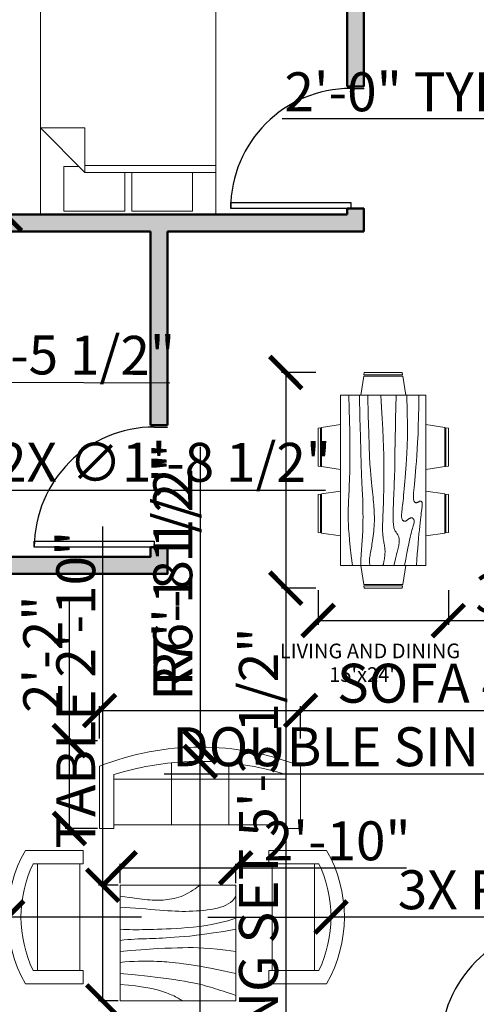
# Model space of a CAD drawing. Units: inches. Extents: x 3147 to 3847, y 1414 to 2207.
# Tile 3 of 7: x 3437 to 3572, y 1561 to 1852. Entities that reach past the tile are written whole.
import ezdxf

# ---------------------------------------------------------------- set-up
doc = ezdxf.new("R2010")
doc.units = ezdxf.units.IN
for name, color, linetype, lineweight in [('A-ANNO-DIMS', 2, 'Continuous', 18), ('A-AREA-IDEN', 7, 'Continuous', 18), ('A-DOOR', 3, 'Continuous', 25), ('A-FURN', 8, 'Continuous', 18), ('A-WALL', 7, 'Continuous', 50)]:
    doc.layers.add(name, color=color, linetype=linetype, lineweight=lineweight)
doc.layers.add('A-WALL-PATT', color=18, linetype='Continuous', lineweight=13, true_color=0x000000)
doc.styles.get("Standard").update_dxf_attribs({"font": 'arial.ttf'})
doc.dimstyles.new('ISO-25', dxfattribs={"dimtxt": 11.5, "dimasz": 9.5, "dimexe": 1.25, "dimexo": 0.625, "dimtad": 1, "dimdec": 0, "dimlunit": 3, "dimtxsty": 'Standard', "dimblk": 'ARCHTICK', "dimcen": 2.5, "dimadec": 0, "dimazin": 0, "dimtfac": 1, "dimtdec": 0, "dimtmove": 0, "dimatfit": 3, "dimfxl": 1, "dimarcsym": 0})

# ---------------------------------------------------------------- blocks, each defined once
blk = doc.blocks.new('*U6')
for p, q in [((0, 0), (0, -100)), ((900, 0), (900, -100))]:
    blk.add_line(p, q)
blk.add_lwpolyline([(0, 0), (0, 900), (43.75, 900), (43.75, 0)], close=True)
blk.add_arc((0, 0), 900, 0, 90)
blk = doc.blocks.new('Sofa - Roundback 7 ft.')
for p, q in [((-12.00002, -32.4421), (-12.00003, -6.5971)), ((11.99997, -32.4421), (11.99998, -6.5971)), ((-36.000027, -34), (-36.000027, -11.4696)), ((35.99998, -34), (35.99998, -11.4696)), ((-35.999844, -13.3819), (35.9998, -13.3819)), ((-36.000027, -32.4421), (35.99998, -32.4421))]:
    blk.add_line(p, q)
for points in [[(-36.000027, -34), (-42.000027, -34), (-42.000027, -8)], [(41.99998, -8), (41.99998, -34), (35.99998, -34)]]:
    blk.add_lwpolyline(points)
for centre, radius, start, end in [((0, -114.25), 114.25, 68.43141, 111.5686), ((-0.00001, -127.1968), 121.1968, 72.72033, 107.2797)]:
    blk.add_arc(centre, radius, start, end)
blk = doc.blocks.new('Table - Square Woodgrain 42 x 42 in.')
blk.add_line((0, -42), (42, -42))
for points in [[(0, -4), (1.704, -4.2172), (3.2358, -4.4188), (4.615, -4.604), (5.8615, -4.7721), (6.9951, -4.9224), (8.0357, -5.0541), (9.0031, -5.1667), (9.9171, -5.2594), (10.7951, -5.3316), (11.6445, -5.3836), (12.4702, -5.4157), (13.277, -5.4283), (14.0698, -5.4217), (14.8535, -5.3964), (15.6331, -5.3526), (16.4133, -5.2908), (17.1986, -5.2103), (17.9913, -5.1062), (18.793, -4.9727), (19.6056, -4.8038), (20.4307, -4.5937), (21.2701, -4.3365), (22.1256, -4.0262), (22.9989, -3.6571), (23.888, -3.2272), (24.7756, -2.7516), (25.6408, -2.2491), (26.4624, -1.7387), (27.2195, -1.2395), (27.891, -0.7703), (28.456, -0.3501), (28.8934, 0.002)], [(0, -42), (0, 0), (42, 0), (42, -42)], [(0, -8), (1.8203, -8.1001), (3.6741, -8.2149), (5.5411, -8.3408), (7.4011, -8.4741), (9.2339, -8.6112), (11.0193, -8.7484), (12.7371, -8.8821), (14.3671, -9.0086), (15.8954, -9.1246), (17.3337, -9.2278), (18.6997, -9.3159), (20.0116, -9.387), (21.2871, -9.4389), (22.5442, -9.4696), (23.8008, -9.477), (25.0749, -9.459), (26.3791, -9.4137), (27.7049, -9.3403), (29.0383, -9.2382), (30.3655, -9.1068), (31.6728, -8.9455), (32.9461, -8.7535), (34.1717, -8.5304), (35.3358, -8.2756), (36.4268, -7.9863), (37.443, -7.6521), (38.3849, -7.2603), (39.253, -6.7986), (40.048, -6.2542), (40.7705, -5.6147), (41.421, -4.8674), (42, -4)], [(42, -12), (39.1784, -12.8621), (36.4519, -13.5654), (33.8246, -14.1294), (31.3004, -14.5731), (28.8832, -14.9161), (26.577, -15.1775), (24.3858, -15.3768), (22.3136, -15.5332), (20.3622, -15.6632), (18.5254, -15.7718), (16.7947, -15.8612), (15.1618, -15.9338), (13.6183, -15.9916), (12.1558, -16.0369), (10.7659, -16.0718), (9.4403, -16.0987), (8.1703, -16.1191), (6.9461, -16.1325), (5.7577, -16.1377), (4.595, -16.1335), (3.4479, -16.1188), (2.3064, -16.0924), (1.1604, -16.0532), (0, -16)], [(42, -16), (37.6529, -16.7365), (33.8802, -17.329), (30.6179, -17.7961), (27.8015, -18.1561), (25.3668, -18.4275), (23.2497, -18.6288), (21.3859, -18.7785), (19.7111, -18.8949), (18.1693, -18.9939), (16.7375, -19.0795), (15.401, -19.1534), (14.1449, -19.217), (12.9544, -19.2717), (11.8148, -19.3191), (10.7113, -19.3606), (9.6291, -19.3976), (8.5534, -19.4323), (7.47, -19.4689), (6.3643, -19.5122), (5.222, -19.5672), (4.0288, -19.6386), (2.7703, -19.7313), (1.4321, -19.8501), (0, -20)], [(0, -24), (3.9243, -23.6805), (7.4766, -23.4138), (10.6891, -23.1954), (13.5943, -23.0205), (16.2247, -22.8847), (18.6125, -22.7832), (20.7903, -22.7116), (22.7903, -22.6651), (24.6563, -22.642), (26.4764, -22.6507), (28.35, -22.7024), (30.3766, -22.8084), (32.6555, -22.98), (35.2861, -23.2283), (38.3678, -23.5645), (42, -24)], [(42, -32), (37.392, -31.017), (33.4585, -30.2231), (30.1291, -29.5949), (27.3334, -29.109), (25.0009, -28.742), (23.0612, -28.4707), (21.4439, -28.2716), (20.0786, -28.1215), (18.8998, -28.0002), (17.8609, -27.9014), (16.9206, -27.8219), (16.0371, -27.7588), (15.1691, -27.709), (14.2748, -27.6693), (13.3128, -27.6368), (12.2415, -27.6083), (11.0295, -27.5824), (9.6867, -27.5643), (8.233, -27.5608), (6.6884, -27.5787), (5.0728, -27.6248), (3.4062, -27.7058), (1.7086, -27.8286), (0, -28)], [(0, -32), (5.4026, -32.5358), (9.9494, -33.019), (13.7424, -33.4553), (16.8834, -33.8505), (19.4743, -34.2106), (21.6171, -34.5413), (23.4136, -34.8486), (24.9657, -35.1382), (26.3614, -35.4156), (27.6332, -35.6841), (28.7995, -35.9467), (29.8788, -36.2064), (30.8897, -36.4661), (31.8507, -36.7288), (32.7802, -36.9973), (33.6968, -37.2747), (34.6175, -37.5635), (35.5531, -37.8651), (36.5128, -38.1805), (37.506, -38.5108), (38.5421, -38.8568), (39.6302, -39.2197), (40.7797, -39.6004), (42, -40)], [(0, -36), (3.0098, -36.2857), (5.5354, -36.5643), (7.6368, -36.8359), (9.374, -37.1009), (10.807, -37.3597), (11.9957, -37.6126), (13.0002, -37.8599), (13.8804, -38.102), (14.6874, -38.3393), (15.4365, -38.5729), (16.1338, -38.8041), (16.7858, -39.0341), (17.3987, -39.264), (17.9787, -39.4952), (18.5322, -39.7288), (19.0655, -39.9662), (19.5832, -40.2081), (20.0842, -40.4544), (20.5657, -40.7046), (21.0249, -40.9581), (21.459, -41.2144), (21.8653, -41.4731), (22.2409, -41.7335), (22.5831, -41.9951)]]:
    blk.add_lwpolyline(points)
blk = doc.blocks.new('Dining Set - 36 x 72 in.')
for p, q in [((-22.2343, 26.00059), (-23.4847, 17.99762)), ((-22.2304, 26), (-5.7608, 26)), ((-22, 27.5), (-22.1562, 26.50042)), ((-5.8416, 26.5), (-22.1534, 26.5)), ((-22, 27.5), (-6, 27.5)), ((-5.8437, 26.49966), (-6, 27.5)), ((-4.5152, 17.99762), (-5.7655, 25.99926)), ((5.7657, 26.00059), (4.5153, 17.99762)), ((5.7696, 26), (22.2392, 26)), ((6, 27.5), (5.8438, 26.50042)), ((22.1584, 26.5), (5.8466, 26.5)), ((6, 27.5), (22, 27.5)), ((22.1563, 26.49966), (22, 27.5)), ((23.4848, 17.99762), (22.2345, 25.99926)), ((36, 18), (-36, 18)), ((-36, 18), (-36, -18)), ((36, -18), (36, 18)), ((-44.0006, 8.23428), (-35.9976, 9.48474)), ((44.0006, 8.23428), (35.9976, 9.48474)), ((-45.5, 8), (-44.5004, 8.15617)), ((-45.5, 8), (-45.5, -8)), ((-44.5, -8.15843), (-44.5, 8.15338)), ((-44, 8.23041), (-44, -8.23915)), ((44, 8.23041), (44, -8.23915)), ((44.5, -8.15843), (44.5, 8.15338)), ((45.5, 8), (44.5005, 8.15617)), ((45.5, 8), (45.5, -8)), ((-44.4997, -8.15631), (-45.5, -8)), ((-35.9976, -9.48476), (-43.9993, -8.2345)), ((35.9976, -9.48476), (43.9993, -8.2345)), ((44.4997, -8.15631), (45.5, -8)), ((-36, -18), (36, -18)), ((-22.2343, -26.0006), (-23.4847, -17.99762)), ((-4.5152, -17.99762), (-5.7655, -25.99928)), ((5.7657, -26.0006), (4.5153, -17.99762)), ((23.4848, -17.99762), (22.2345, -25.99928)), ((-22.2304, -26), (-5.7608, -26)), ((-22, -27.5), (-22.1562, -26.50044)), ((-5.8416, -26.5), (-22.1534, -26.5)), ((-22, -27.5), (-6, -27.5)), ((-5.8437, -26.49967), (-6, -27.5)), ((5.7696, -26), (22.2392, -26)), ((6, -27.5), (5.8438, -26.50044)), ((22.1584, -26.5), (5.8466, -26.5)), ((6, -27.5), (22, -27.5)), ((22.1563, -26.49967), (22, -27.5))]:
    blk.add_line(p, q)
for points in [[(-36, 15), (-31.1772, 14.97754), (-26.8079, 14.91406), (-22.8538, 14.81543), (-19.276, 14.6875), (-16.0362, 14.53613), (-13.0957, 14.36718), (-10.4159, 14.18652), (-7.9583, 14), (-5.6904, 13.81315), (-3.6035, 13.63021), (-1.6954, 13.45508), (0.0365, 13.29166), (1.5945, 13.14388), (2.9811, 13.01562), (4.1988, 12.9108), (5.25, 12.83333), (6.1393, 12.78613), (6.8802, 12.76823), (7.4883, 12.77767), (7.9792, 12.8125), (8.3685, 12.87077), (8.6719, 12.95052), (8.9049, 13.0498), (9.0833, 13.16666), (9.2205, 13.29899), (9.3216, 13.44401), (9.3895, 13.59879), (9.4271, 13.76041), (9.4373, 13.92594), (9.4232, 14.09245), (9.3875, 14.257), (9.3333, 14.41666), (9.2638, 14.56917), (9.1836, 14.71484), (9.0975, 14.85465), (9.0104, 14.98958), (8.9272, 15.1206), (8.8529, 15.2487), (8.7922, 15.37483), (8.75, 15.5), (8.7305, 15.62467), (8.7344, 15.74739), (8.7617, 15.86621), (8.8125, 15.97916), (8.8867, 16.08431), (8.9844, 16.17968), (9.1055, 16.26334), (9.25, 16.33333), (9.4189, 16.38802), (9.6172, 16.42708), (9.8506, 16.45052), (10.125, 16.45833), (10.4463, 16.45052), (10.8203, 16.42708), (11.2529, 16.38802), (11.75, 16.33333), (12.3184, 16.26318), (12.9694, 16.17838), (13.7151, 16.07991), (14.5677, 15.96875), (15.5395, 15.84586), (16.6426, 15.71224), (17.8893, 15.56884), (19.2917, 15.41666), (20.859, 15.25667), (22.5879, 15.08984), (24.4721, 14.91715), (26.5052, 14.73958), (28.6809, 14.5581), (30.9929, 14.3737), (33.4347, 14.18733), (36, 14)], [(-36, 10), (-28.9766, 10.14274), (-23.1725, 10.20442), (-18.4241, 10.19775), (-14.5677, 10.13541), (-11.4399, 10.03011), (-8.877, 9.89453), (-6.7154, 9.74137), (-4.7917, 9.58333), (-2.9698, 9.43082), (-1.2246, 9.28515), (0.4415, 9.14534), (2.026, 9.01041), (3.5266, 8.87939), (4.9408, 8.7513), (6.266, 8.62516), (7.5, 8.5), (8.6411, 8.37549), (9.6914, 8.2539), (10.6538, 8.13818), (11.5312, 8.03125), (12.3267, 7.93603), (13.043, 7.85547), (13.6831, 7.79248), (14.25, 7.75), (14.7471, 7.7303), (15.1797, 7.73307), (15.5537, 7.75732), (15.875, 7.80208), (16.1494, 7.86637), (16.3828, 7.94922), (16.5811, 8.04964), (16.75, 8.16666), (16.8944, 8.29915), (17.0143, 8.44531), (17.1089, 8.60319), (17.1771, 8.77083), (17.218, 8.94629), (17.2305, 9.1276), (17.2137, 9.31282), (17.1667, 9.5), (17.0895, 9.6875), (16.987, 9.875), (16.8649, 10.0625), (16.7292, 10.25), (16.5856, 10.4375), (16.4401, 10.625), (16.2985, 10.8125), (16.1667, 11), (16.05, 11.18733), (15.9518, 11.3737), (15.8752, 11.5581), (15.8229, 11.73958), (15.798, 11.91715), (15.8034, 12.08984), (15.842, 12.25667), (15.9167, 12.41666), (16.0295, 12.56836), (16.1784, 12.70833), (16.3605, 12.83268), (16.5729, 12.9375), (16.8127, 13.01888), (17.0768, 13.07291), (17.3625, 13.0957), (17.6667, 13.08333), (17.9894, 13.03312), (18.3418, 12.94726), (18.7382, 12.82918), (19.1927, 12.68229), (19.7195, 12.51001), (20.3327, 12.31575), (21.0465, 12.10294), (21.875, 11.875), (22.8357, 11.63354), (23.959, 11.37304), (25.2786, 11.08618), (26.8282, 10.76562), (28.6414, 10.40405), (30.752, 9.99414), (33.1936, 9.52856), (36, 9)], [(-36, 5.5), (-30.7157, 5.3348), (-26.069, 5.20963), (-21.9946, 5.11767), (-18.4271, 5.05208), (-15.3009, 5.00602), (-12.5508, 4.97265), (-10.1112, 4.94515), (-7.9167, 4.91666), (-5.909, 4.88167), (-4.0586, 4.83984), (-2.3429, 4.79215), (-0.7396, 4.73958), (0.7739, 4.6831), (2.22, 4.6237), (3.6213, 4.56233), (5, 4.5), (6.373, 4.43782), (7.7344, 4.3776), (9.0723, 4.32129), (10.375, 4.27083), (11.6309, 4.22819), (12.8281, 4.19531), (13.9551, 4.17415), (15, 4.16666), (15.954, 4.17448), (16.819, 4.19791), (17.6001, 4.23698), (18.3021, 4.29166), (18.9299, 4.36198), (19.4883, 4.44791), (19.9823, 4.54948), (20.4167, 4.66666), (20.7969, 4.79899), (21.1302, 4.94401), (21.4245, 5.09879), (21.6875, 5.26041), (21.9271, 5.42594), (22.1511, 5.59245), (22.3672, 5.757), (22.5834, 5.91666), (22.8065, 6.06868), (23.0404, 6.21093), (23.2879, 6.34147), (23.5521, 6.45833), (23.8358, 6.55957), (24.142, 6.64323), (24.4735, 6.70735), (24.8334, 6.75), (25.2235, 6.76969), (25.642, 6.76692), (26.0858, 6.74267), (26.5521, 6.69791), (27.0379, 6.63362), (27.5404, 6.55078), (28.0565, 6.45036), (28.5834, 6.33333), (29.1242, 6.19987), (29.7071, 6.04687), (30.3661, 5.87044), (31.1354, 5.66666), (32.0493, 5.43164), (33.142, 5.16146), (34.4475, 4.85221), (36, 4.5)], [(-36, -1), (-30.7915, -0.6591), (-26.0195, -0.38216), (-21.6519, -0.16284), (-17.6563, 0.00521), (-14.0005, 0.12833), (-10.6523, 0.21289), (-7.5796, 0.26522), (-4.75, 0.29166), (-2.134, 0.29793), (0.2878, 0.28711), (2.5317, 0.26163), (4.6146, 0.22396), (6.5529, 0.17651), (8.3633, 0.12174), (10.0623, 0.06209), (11.6667, 0), (13.1899, -0.06201), (14.6341, -0.1211), (15.9982, -0.17432), (17.2813, -0.21875), (18.4823, -0.25147), (19.6003, -0.26953), (20.6343, -0.27002), (21.5834, -0.25), (22.4481, -0.20768), (23.2357, -0.14584), (23.9549, -0.06836), (24.6146, 0.02083), (25.2235, 0.11784), (25.7904, 0.21875), (26.3241, 0.31966), (26.8334, 0.41666), (27.3265, 0.50618), (27.8099, 0.58593), (28.2894, 0.65397), (28.7709, 0.70833), (29.2601, 0.74707), (29.763, 0.76823), (30.2855, 0.76985), (30.8334, 0.75), (31.4088, 0.70784), (31.9994, 0.64713), (32.589, 0.57275), (33.1615, 0.48958), (33.7008, 0.4025), (34.1908, 0.3164), (34.6153, 0.23616), (34.9584, 0.16666), (35.2099, 0.11165), (35.3848, 0.07031), (35.504, 0.04069), (35.5886, 0.02083), (35.6594, 0.00879), (35.7377, 0.0026), (35.8442, 0.00032), (36, 0)], [(-36, -6.5), (-27.1843, -6.31267), (-20.084, -6.1263), (-14.469, -5.9419), (-10.1094, -5.76042), (-6.7752, -5.58285), (-4.2363, -5.41016), (-2.2629, -5.24333), (-0.625, -5.08334), (0.8708, -4.93099), (2.2715, -4.78646), (3.5872, -4.64974), (4.8281, -4.52084), (6.0046, -4.39974), (7.127, -4.28646), (8.2053, -4.18099), (9.25, -4.08334), (10.2705, -3.99382), (11.2734, -3.91407), (12.2647, -3.84603), (13.25, -3.79167), (14.2354, -3.75293), (15.2266, -3.73177), (16.2295, -3.73015), (17.25, -3.75), (18.2912, -3.79248), (19.3451, -3.85547), (20.4009, -3.93604), (21.4479, -4.03125), (22.4754, -4.13819), (23.4727, -4.25391), (24.4289, -4.37549), (25.3334, -4.5), (26.1785, -4.62492), (26.9694, -4.74935), (27.7145, -4.87281), (28.4219, -4.99479), (29.1, -5.11483), (29.7572, -5.23242), (30.4016, -5.34709), (31.0417, -5.45834), (31.6837, -5.56437), (32.3262, -5.65821), (32.9658, -5.73153), (33.599, -5.77604), (34.2224, -5.78345), (34.8327, -5.74545), (35.4264, -5.65373), (36, -5.5)], [(-36, -10), (-26.4022, -9.81299), (-18.4675, -9.62891), (-11.9839, -9.45069), (-6.7396, -9.28125), (-2.5226, -9.12354), (0.8789, -8.98047), (3.6769, -8.85498), (6.0833, -8.75), (8.2767, -8.66765), (10.3021, -8.60677), (12.1712, -8.56543), (13.8958, -8.54167), (15.4876, -8.53353), (16.9583, -8.53907), (18.3197, -8.55632), (19.5834, -8.58334), (20.7616, -8.61841), (21.8685, -8.66081), (22.9188, -8.71004), (23.9271, -8.76563), (24.9081, -8.82707), (25.8763, -8.89388), (26.8465, -8.96558), (27.8334, -9.04167), (28.8474, -9.12118), (29.8828, -9.20117), (30.93, -9.27824), (31.9792, -9.34896), (33.0205, -9.40991), (34.0443, -9.45768), (35.0407, -9.48885), (36, -9.5)], [(-36, -14.5), (-30.0881, -14.33513), (-25.0332, -14.21224), (-20.7312, -14.12647), (-17.0781, -14.07292), (-13.97, -14.04671), (-11.3027, -14.04297), (-8.9724, -14.05681), (-6.875, -14.08334), (-4.9224, -14.11833), (-3.0905, -14.16016), (-1.3709, -14.20785), (0.2448, -14.26042), (1.7647, -14.3169), (3.1973, -14.3763), (4.5507, -14.43767), (5.8333, -14.5), (7.0554, -14.5621), (8.235, -14.62175), (9.3922, -14.67652), (10.5469, -14.72396), (11.7192, -14.76164), (12.929, -14.78711), (14.1965, -14.79794), (15.5417, -14.79167), (16.9933, -14.76424), (18.6152, -14.70508), (20.4804, -14.60197), (22.6615, -14.44271), (25.2312, -14.21509), (28.2624, -13.9069), (31.8277, -13.50594), (36, -13)]]:
    blk.add_lwpolyline(points)
blk = doc.blocks.new('Bed - Queen')
for p, q in [((0, -80.00003), (0, 0)), ((0, 0), (59.99999, 0)), ((59.99999, 0), (59.99999, -80.00003)), ((7.99999, -1.2), (28.79998, -1.2)), ((7.99999, -14.4), (7.99999, -1.2)), ((28.79998, -1.2), (28.79998, -14.4)), ((31.19999, -1.2), (51.99999, -1.2)), ((31.19999, -14.4), (31.19999, -1.2)), ((51.99999, -1.2), (51.99999, -16.4)), ((0, -14.4), (44.8, -14.4)), ((44.8, -16.8), (0, -16.8)), ((59.99999, -29.6), (44.8, -14.4)), ((44.8, -14.4), (44.8, -29.6)), ((51.99999, -16.4), (46.79936, -16.4)), ((44.8, -29.6), (59.99999, -29.6)), ((59.99999, -80.00003), (0, -80.00003))]:
    blk.add_line(p, q)
blk = doc.blocks.new('Sofa - Roundback Loveseat 5 ft.')
for p, q in [((0, -32.44198), (0, -5.99998)), ((-24, -33.99998), (-24, -11.46958)), ((24.00004, -33.99998), (24.00004, -11.46958)), ((-23.9998, -13.38178), (23.99986, -13.38178)), ((-24, -32.44198), (24.00004, -32.44198))]:
    blk.add_line(p, q)
for points in [[(-24, -33.99998), (-30, -33.99998), (-30, -7.99998)], [(30.00004, -7.99998), (30.00004, -33.99998), (24.00004, -33.99998)]]:
    blk.add_lwpolyline(points)
for centre, radius, start, end in [((0, -60.24998), 60.24998, 60.13715, 119.8628), ((0, -61.38438), 55.38444, 64.32083, 115.6792)]:
    blk.add_arc(centre, radius, start, end)
blk = doc.blocks.new('_ArchTick')
at = {"color": 0, "linetype": 'ByBlock', "const_width": 0.15}
blk.add_lwpolyline([(-0.5, -0.5), (0.5, 0.5)], dxfattribs=at)
blk = doc.blocks.new('*D35')
at = {"layer": 'A-ANNO-DIMS', "color": 0, "lineweight": -2, "transparency": 16777216}
for p, q in [((3442.6, 1863.12), (3431.61, 1863.12)), ((3432.86, 1863.12), (3432.86, 1794.05)), ((3442.6, 1794.05), (3431.61, 1794.05))]:
    blk.add_line(p, q, dxfattribs=at)
at = {"layer": 'Defpoints', "color": 0, "transparency": 16777216}
for p in [(3443.22, 1863.12), (3432.86, 1794.05), (3443.22, 1794.05)]:
    blk.add_point(p, dxfattribs=at)
at = {"layer": 'A-ANNO-DIMS', "color": 0, "lineweight": -2, "transparency": 16777216, "xscale": 9.5, "yscale": 9.5, "zscale": 9.5}
for p, rotation in [((3432.86, 1863.12), 90), ((3432.86, 1794.05), 270)]:
    blk.add_blockref('_ArchTick', p, dxfattribs=dict(at, rotation=rotation))
at = {"layer": 'A-ANNO-DIMS', "color": 0, "transparency": 16777216, "insert": (3426.36, 1828.59), "char_height": 11.5, "attachment_point": 5, "rotation": 90}
blk.add_mtext('BED 5\'-9"', dxfattribs=at)
blk = doc.blocks.new('*D38')
at = {"layer": 'A-ANNO-DIMS', "color": 0, "lineweight": -2, "transparency": 16777216}
for p, q in [((3595.65, 1822.28), (3514.6, 1822.28)), ((3595.65, 1817), (3595.65, 1823.53)), ((3619.7, 1822.28), (3595.65, 1822.28)), ((3619.7, 1817), (3619.7, 1823.53))]:
    blk.add_line(p, q, dxfattribs=at)
at = {"layer": 'Defpoints', "color": 0, "transparency": 16777216}
for p in [(3595.65, 1822.28), (3595.65, 1816.38), (3619.7, 1816.38)]:
    blk.add_point(p, dxfattribs=at)
at = {"layer": 'A-ANNO-DIMS', "color": 0, "lineweight": -2, "transparency": 16777216, "xscale": 9.5, "yscale": 9.5, "zscale": 9.5, "rotation": 180}
blk.add_blockref('_ArchTick', (3595.65, 1822.28), dxfattribs=at)
at = {"layer": 'A-ANNO-DIMS', "color": 0, "lineweight": -2, "transparency": 16777216, "xscale": 9.5, "yscale": 9.5, "zscale": 9.5}
blk.add_blockref('_ArchTick', (3619.7, 1822.28), dxfattribs=at)
at = {"layer": 'A-ANNO-DIMS', "color": 0, "transparency": 16777216, "insert": (3550.37, 1828.78), "char_height": 11.5, "attachment_point": 5}
blk.add_mtext('2\'-0" TYP.', dxfattribs=at)
blk = doc.blocks.new('*D41')
at = {"layer": 'A-ANNO-DIMS', "color": 0, "lineweight": -2, "transparency": 16777216}
for p, q in [((3460.68, 1639.4), (3460.68, 1648.92)), ((3460.68, 1647.67), (3520.02, 1647.67)), ((3520.02, 1639.4), (3520.02, 1648.92)), ((3520.02, 1647.67), (3645.23, 1647.67))]:
    blk.add_line(p, q, dxfattribs=at)
at = {"layer": 'Defpoints', "color": 0, "transparency": 16777216}
for p in [(3520.02, 1647.67), (3460.68, 1638.77), (3520.02, 1638.77)]:
    blk.add_point(p, dxfattribs=at)
at = {"layer": 'A-ANNO-DIMS', "color": 0, "lineweight": -2, "transparency": 16777216, "xscale": 9.5, "yscale": 9.5, "zscale": 9.5, "rotation": 180}
blk.add_blockref('_ArchTick', (3460.68, 1647.67), dxfattribs=at)
at = {"layer": 'A-ANNO-DIMS', "color": 0, "lineweight": -2, "transparency": 16777216, "xscale": 9.5, "yscale": 9.5, "zscale": 9.5}
blk.add_blockref('_ArchTick', (3520.02, 1647.67), dxfattribs=at)
at = {"layer": 'A-ANNO-DIMS', "color": 0, "transparency": 16777216, "insert": (3587.38, 1654.25), "char_height": 11.5, "attachment_point": 5}
blk.add_mtext('SOFA 4\'-11 1/2"', dxfattribs=at)
blk = doc.blocks.new('*D42')
at = {"layer": 'A-ANNO-DIMS', "color": 0, "lineweight": -2, "transparency": 16777216}
for p, q in [((3451.77, 1638.77), (3451.77, 1680.29)), ((3460.05, 1638.77), (3450.52, 1638.77)), ((3451.77, 1612.86), (3451.77, 1638.77)), ((3460.05, 1612.86), (3450.52, 1612.86))]:
    blk.add_line(p, q, dxfattribs=at)
at = {"layer": 'Defpoints', "color": 0, "transparency": 16777216}
for p in [(3451.77, 1638.77), (3460.68, 1638.77), (3460.68, 1612.86)]:
    blk.add_point(p, dxfattribs=at)
at = {"layer": 'A-ANNO-DIMS', "color": 0, "lineweight": -2, "transparency": 16777216, "xscale": 9.5, "yscale": 9.5, "zscale": 9.5}
for p, rotation in [((3451.77, 1638.77), 90), ((3451.77, 1612.86), 270)]:
    blk.add_blockref('_ArchTick', p, dxfattribs=dict(at, rotation=rotation))
at = {"layer": 'A-ANNO-DIMS', "color": 0, "transparency": 16777216, "insert": (3445.37, 1664.28), "char_height": 11.5, "attachment_point": 5, "rotation": 90}
blk.add_mtext('2\'-2"', dxfattribs=at)
blk = doc.blocks.new('*D43')
at = {"layer": 'A-ANNO-DIMS', "color": 0, "lineweight": -2, "transparency": 16777216}
for p, q in [((3461.63, 1596.11), (3461.63, 1702.01)), ((3466.13, 1596.11), (3460.38, 1596.11)), ((3461.63, 1561.97), (3461.63, 1596.11)), ((3466.13, 1561.97), (3460.38, 1561.97))]:
    blk.add_line(p, q, dxfattribs=at)
at = {"layer": 'Defpoints', "color": 0, "transparency": 16777216}
for p in [(3461.63, 1596.11), (3466.75, 1596.11), (3466.75, 1561.97)]:
    blk.add_point(p, dxfattribs=at)
at = {"layer": 'A-ANNO-DIMS', "color": 0, "lineweight": -2, "transparency": 16777216, "xscale": 9.5, "yscale": 9.5, "zscale": 9.5}
for p, rotation in [((3461.63, 1596.11), 90), ((3461.63, 1561.97), 270)]:
    blk.add_blockref('_ArchTick', p, dxfattribs=dict(at, rotation=rotation))
at = {"layer": 'A-ANNO-DIMS', "color": 0, "transparency": 16777216, "insert": (3455.13, 1653.81), "char_height": 11.5, "attachment_point": 5, "rotation": 90}
blk.add_mtext('TABLE 2\'-10"', dxfattribs=at)
blk = doc.blocks.new('*D44')
at = {"layer": 'A-ANNO-DIMS', "color": 0, "lineweight": -2, "transparency": 16777216}
for p, q in [((3466.75, 1596.73), (3466.75, 1602.48)), ((3466.75, 1601.23), (3500.88, 1601.23)), ((3500.88, 1596.73), (3500.88, 1602.48)), ((3500.88, 1601.23), (3551.33, 1601.23))]:
    blk.add_line(p, q, dxfattribs=at)
at = {"layer": 'Defpoints', "color": 0, "transparency": 16777216}
for p in [(3500.88, 1601.23), (3466.75, 1596.11), (3500.88, 1596.11)]:
    blk.add_point(p, dxfattribs=at)
at = {"layer": 'A-ANNO-DIMS', "color": 0, "lineweight": -2, "transparency": 16777216, "xscale": 9.5, "yscale": 9.5, "zscale": 9.5, "rotation": 180}
blk.add_blockref('_ArchTick', (3466.75, 1601.23), dxfattribs=at)
at = {"layer": 'A-ANNO-DIMS', "color": 0, "lineweight": -2, "transparency": 16777216, "xscale": 9.5, "yscale": 9.5, "zscale": 9.5}
blk.add_blockref('_ArchTick', (3500.88, 1601.23), dxfattribs=at)
at = {"layer": 'A-ANNO-DIMS', "color": 0, "transparency": 16777216, "insert": (3530.86, 1607.73), "char_height": 11.5, "attachment_point": 5}
blk.add_mtext('2\'-10"', dxfattribs=at)
blk = doc.blocks.new('*D45')
at = {"layer": 'A-ANNO-DIMS', "color": 0, "lineweight": -2, "transparency": 16777216}
for p, q in [((3668.72, 1622.4), (3668.72, 1630.17)), ((3716.33, 1622.4), (3716.33, 1630.17)), ((3668.72, 1628.92), (3479.75, 1628.92)), ((3716.33, 1628.92), (3668.72, 1628.92))]:
    blk.add_line(p, q, dxfattribs=at)
at = {"layer": 'Defpoints', "color": 0, "transparency": 16777216}
for p in [(3668.72, 1628.92), (3668.72, 1621.78), (3716.33, 1621.78)]:
    blk.add_point(p, dxfattribs=at)
at = {"layer": 'A-ANNO-DIMS', "color": 0, "lineweight": -2, "transparency": 16777216, "xscale": 9.5, "yscale": 9.5, "zscale": 9.5, "rotation": 180}
blk.add_blockref('_ArchTick', (3668.72, 1628.92), dxfattribs=at)
at = {"layer": 'A-ANNO-DIMS', "color": 0, "lineweight": -2, "transparency": 16777216, "xscale": 9.5, "yscale": 9.5, "zscale": 9.5}
blk.add_blockref('_ArchTick', (3716.33, 1628.92), dxfattribs=at)
at = {"layer": 'A-ANNO-DIMS', "color": 0, "transparency": 16777216, "insert": (3569.49, 1635.5), "char_height": 11.5, "attachment_point": 5}
blk.add_mtext('DOUBLE SINK 3\'-11 1/2"', dxfattribs=at)
blk = doc.blocks.new('*D49')
at = {"layer": 'A-ANNO-DIMS', "color": 0, "lineweight": -2, "transparency": 16777216}
for p, q in [((3524.58, 1747.43), (3514.41, 1747.43)), ((3515.66, 1747.43), (3515.66, 1683.78)), ((3524.58, 1683.78), (3514.41, 1683.78)), ((3515.66, 1683.78), (3515.66, 1519.84))]:
    blk.add_line(p, q, dxfattribs=at)
at = {"layer": 'Defpoints', "color": 0, "transparency": 16777216}
for p in [(3525.21, 1747.43), (3515.66, 1683.78), (3525.21, 1683.78)]:
    blk.add_point(p, dxfattribs=at)
at = {"layer": 'A-ANNO-DIMS', "color": 0, "lineweight": -2, "transparency": 16777216, "xscale": 9.5, "yscale": 9.5, "zscale": 9.5}
for p, rotation in [((3515.66, 1747.43), 90), ((3515.66, 1683.78), 270)]:
    blk.add_blockref('_ArchTick', p, dxfattribs=dict(at, rotation=rotation))
at = {"layer": 'A-ANNO-DIMS', "color": 0, "transparency": 16777216, "insert": (3509.09, 1597.06), "char_height": 11.5, "attachment_point": 5, "rotation": 90}
blk.add_mtext('DINING SET 5\'-3 1/2"', dxfattribs=at)
blk = doc.blocks.new('*D50')
at = {"layer": 'A-ANNO-DIMS', "color": 0, "lineweight": -2, "transparency": 16777216}
for p, q in [((3525.21, 1683.16), (3525.21, 1672.98)), ((3563.68, 1683.16), (3563.68, 1672.98)), ((3525.21, 1674.23), (3563.68, 1674.23)), ((3563.68, 1674.23), (3631.79, 1674.23))]:
    blk.add_line(p, q, dxfattribs=at)
at = {"layer": 'Defpoints', "color": 0, "transparency": 16777216}
for p in [(3525.21, 1683.78), (3563.68, 1683.78), (3563.68, 1674.23)]:
    blk.add_point(p, dxfattribs=at)
at = {"layer": 'A-ANNO-DIMS', "color": 0, "lineweight": -2, "transparency": 16777216, "xscale": 9.5, "yscale": 9.5, "zscale": 9.5, "rotation": 180}
blk.add_blockref('_ArchTick', (3525.21, 1674.23), dxfattribs=at)
at = {"layer": 'A-ANNO-DIMS', "color": 0, "lineweight": -2, "transparency": 16777216, "xscale": 9.5, "yscale": 9.5, "zscale": 9.5}
blk.add_blockref('_ArchTick', (3563.68, 1674.23), dxfattribs=at)
at = {"layer": 'A-ANNO-DIMS', "color": 0, "transparency": 16777216, "insert": (3602.48, 1680.81), "char_height": 11.5, "attachment_point": 5}
blk.add_mtext('3\'-2 1/2"', dxfattribs=at)
blk = doc.blocks.new('*D51')
at = {"layer": 'A-ANNO-DIMS', "color": 0, "lineweight": -2, "transparency": 16777216}
for p, q in [((3383.32, 1713.42), (3383.48, 1746.09)), ((3383.47, 1744.84), (3413.15, 1744.7)), ((3413, 1713.28), (3413.15, 1745.95)), ((3413.15, 1744.7), (3481.46, 1744.38))]:
    blk.add_line(p, q, dxfattribs=at)
at = {"layer": 'Defpoints', "color": 0, "transparency": 16777216}
for p in [(3413.15, 1744.7), (3383.32, 1712.8), (3412.99, 1712.65)]:
    blk.add_point(p, dxfattribs=at)
at = {"layer": 'A-ANNO-DIMS', "color": 0, "lineweight": -2, "transparency": 16777216, "xscale": 9.5, "yscale": 9.5, "zscale": 9.5}
for p, rotation in [((3383.47, 1744.84), 179.7281677872788), ((3413.15, 1744.7), 359.7281677872788)]:
    blk.add_blockref('_ArchTick', p, dxfattribs=dict(at, rotation=rotation))
at = {"layer": 'A-ANNO-DIMS', "color": 0, "transparency": 16777216, "insert": (3452.08, 1751.09), "char_height": 11.5, "attachment_point": 5, "rotation": 359.7282}
blk.add_mtext('2\'-5 1/2"', dxfattribs=at)
blk = doc.blocks.new('*D94')
at = {"layer": 'A-ANNO-DIMS', "color": 0, "lineweight": -2, "transparency": 16777216}
for p in [(3392.74, 1712.66), (3527.42, 1712.6)]:
    blk.add_line(p, (3412.99, 1712.65), dxfattribs=at)
at = {"layer": 'Defpoints', "color": 0, "transparency": 16777216}
for p in [(3392.74, 1712.66), (3412.99, 1712.65)]:
    blk.add_point(p, dxfattribs=at)
at = {"layer": 'A-ANNO-DIMS', "color": 0, "lineweight": -2, "transparency": 16777216, "xscale": 9.5, "yscale": 9.5, "zscale": 9.5}
for p, rotation in [((3392.74, 1712.66), 359.9757507078119), ((3412.99, 1712.65), 179.9757507078119)]:
    blk.add_blockref('_ArchTick', p, dxfattribs=dict(at, rotation=rotation))
at = {"layer": 'A-ANNO-DIMS', "color": 0, "transparency": 16777216, "insert": (3479.71, 1719.44), "char_height": 11.5, "attachment_point": 5, "rotation": 359.9758}
blk.add_mtext('2X ∅1\'-8 1/2"', dxfattribs=at)
blk = doc.blocks.new('*D95')
at = {"layer": 'A-ANNO-DIMS', "color": 0, "lineweight": -2, "transparency": 16777216}
for p in [(3490.35, 1721.27), (3490.35, 1547.02)]:
    blk.add_line(p, (3490.35, 1632.65), dxfattribs=at)
at = {"layer": 'Defpoints', "color": 0, "transparency": 16777216}
for p in [(3490.35, 1632.65), (3490.35, 1547.02)]:
    blk.add_point(p, dxfattribs=at)
at = {"layer": 'A-ANNO-DIMS', "color": 0, "lineweight": -2, "transparency": 16777216, "xscale": 9.5, "yscale": 9.5, "zscale": 9.5, "rotation": 270}
blk.add_blockref('_ArchTick', (3490.35, 1632.65), dxfattribs=at)
at = {"layer": 'A-ANNO-DIMS', "color": 0, "transparency": 16777216, "insert": (3483.78, 1686.46), "char_height": 11.5, "attachment_point": 5, "rotation": 90}
blk.add_mtext('R7\'-1 1/2"', dxfattribs=at)
blk = doc.blocks.new('*D96')
at = {"layer": 'A-ANNO-DIMS', "color": 0, "lineweight": -2, "transparency": 16777216}
for p in [(3490.35, 1725.51), (3490.35, 1556.16)]:
    blk.add_line(p, (3490.35, 1636.89), dxfattribs=at)
at = {"layer": 'Defpoints', "color": 0, "transparency": 16777216}
for p in [(3490.35, 1636.89), (3490.35, 1556.16)]:
    blk.add_point(p, dxfattribs=at)
at = {"layer": 'A-ANNO-DIMS', "color": 0, "lineweight": -2, "transparency": 16777216, "xscale": 9.5, "yscale": 9.5, "zscale": 9.5, "rotation": 270}
blk.add_blockref('_ArchTick', (3490.35, 1636.89), dxfattribs=at)
at = {"layer": 'A-ANNO-DIMS', "color": 0, "transparency": 16777216, "insert": (3483.78, 1690.7), "char_height": 11.5, "attachment_point": 5, "rotation": 90}
blk.add_mtext('R6\'-8 1/2"', dxfattribs=at)
blk = doc.blocks.new('*D97')
at = {"layer": 'A-ANNO-DIMS', "color": 0, "lineweight": -2, "transparency": 16777216}
for p in [(3320.2, 1586.73), (3473.05, 1586.73)]:
    blk.add_line(p, (3433.52, 1586.73), dxfattribs=at)
at = {"layer": 'Defpoints', "color": 0, "transparency": 16777216}
for p in [(3433.52, 1586.73), (3473.05, 1586.73)]:
    blk.add_point(p, dxfattribs=at)
at = {"layer": 'A-ANNO-DIMS', "color": 0, "lineweight": -2, "transparency": 16777216, "xscale": 9.5, "yscale": 9.5, "zscale": 9.5, "rotation": 359.9999231677337}
blk.add_blockref('_ArchTick', (3433.52, 1586.73), dxfattribs=at)
at = {"layer": 'A-ANNO-DIMS', "color": 0, "transparency": 16777216, "insert": (3367.36, 1593.3), "char_height": 11.5, "attachment_point": 5, "rotation": 359.9999}
blk.add_mtext('3X R3\'-3 1/2"', dxfattribs=at)
blk = doc.blocks.new('*D98')
at = {"layer": 'A-ANNO-DIMS', "color": 0, "lineweight": -2, "transparency": 16777216}
for p in [(3492.69, 1586.73), (3642.35, 1586.73)]:
    blk.add_line(p, (3529.03, 1586.73), dxfattribs=at)
at = {"layer": 'Defpoints', "color": 0, "transparency": 16777216}
for p in [(3492.69, 1586.73), (3529.03, 1586.73)]:
    blk.add_point(p, dxfattribs=at)
at = {"layer": 'A-ANNO-DIMS', "color": 0, "lineweight": -2, "transparency": 16777216, "xscale": 9.5, "yscale": 9.5, "zscale": 9.5, "rotation": 180.0000425795118}
blk.add_blockref('_ArchTick', (3529.03, 1586.73), dxfattribs=at)
at = {"layer": 'A-ANNO-DIMS', "color": 0, "transparency": 16777216, "insert": (3595.19, 1593.3), "char_height": 11.5, "attachment_point": 5, "rotation": 0}
blk.add_mtext('3X R3\'-0 1/2"', dxfattribs=at)

msp = doc.modelspace()

# ---------------------------------------------------------------- hatches: boundary and pattern name
at = {"layer": 'A-WALL-PATT'}
h = msp.add_hatch(color=256, dxfattribs=at)
h.dxf.hatch_style = 1
h.paths.add_polyline_path([(3616.76, 2093.05), (3594.02, 2093.05), (3594.02, 2087.05), (3611.76, 2087.05), (3611.76, 1993.05), (3616.76, 1993.05), (3628.76, 1993.05), (3628.76, 1996.99), (3628.76, 1998.05), (3616.76, 1998.05), (3616.76, 2087.05)])
h.paths.add_polyline_path([(3576.44, 2093.05), (3527.03, 2093.05), (3527.03, 2087.05), (3546.76, 2087.05), (3546.76, 1962.05), (3551.76, 1962.05), (3590.76, 1962.05), (3590.76, 1921.05), (3585.76, 1921.05), (3585.76, 1916.05), (3590.76, 1916.05), (3590.76, 1895.05), (3595.76, 1895.05), (3595.76, 1962.05), (3611.76, 1962.05), (3616.76, 1962.05), (3616.76, 1969.05), (3611.76, 1969.05), (3611.76, 1967.05), (3551.76, 1967.05), (3551.76, 2087.05), (3576.44, 2087.05)])
h.paths.add_polyline_path([(3455.03, 2093.05), (3408.76, 2093.05), (3408.76, 2087.05), (3408.76, 2046.06), (3413.76, 2046.06), (3413.76, 2087.05), (3455.03, 2087.05)])
h.paths.add_polyline_path([(3355.76, 2008.05), (3408.76, 2008.05), (3408.76, 2004.83), (3413.76, 2004.83), (3413.76, 2008.05), (3413.76, 2013.05), (3413.76, 2016.06), (3408.76, 2016.06), (3408.76, 2013.05), (3355.76, 2013.05), (3349.76, 2013.05), (3349.76, 1973.71), (3355.76, 1973.71)])
h.paths.add_polyline_path([(3413.76, 1974.83), (3408.76, 1974.83), (3408.76, 1943.05), (3355.76, 1943.05), (3355.76, 1949.71), (3349.76, 1949.71), (3349.76, 1897.34), (3355.76, 1897.34), (3355.76, 1938.05), (3408.76, 1938.05), (3408.76, 1934.63), (3413.76, 1934.63), (3413.76, 1938.05), (3505.76, 1938.05), (3505.76, 1916.05), (3533.76, 1916.05), (3533.76, 1904.63), (3533.76, 1831.83), (3538.76, 1831.83), (3538.76, 1904.63), (3538.76, 1916.05), (3546.76, 1916.05), (3549.76, 1916.05), (3549.76, 1921.05), (3546.76, 1921.05), (3510.76, 1921.05), (3510.76, 1938.05), (3510.76, 1943.05), (3413.76, 1943.05)])
h.paths.add_polyline_path([(3413.76, 1904.63), (3408.76, 1904.63), (3408.76, 1870.05), (3355.76, 1870.05), (3355.76, 1873.34), (3349.76, 1873.34), (3349.76, 1865.05), (3355.76, 1865.05), (3408.76, 1865.05), (3408.76, 1863.11), (3409.83, 1863.11), (3413.76, 1863.11)], flags=17)
h.paths.add_polyline_path([(3538.76, 1795.83), (3533.76, 1795.83), (3533.76, 1794.05), (3413.76, 1794.05), (3413.76, 1833.11), (3408.76, 1833.11), (3408.76, 1794.05), (3355.76, 1794.05), (3349.76, 1794.05), (3349.76, 1776.88), (3355.76, 1776.88), (3355.76, 1789.05), (3413.76, 1789.05), (3475.76, 1789.05), (3475.76, 1731.91), (3480.76, 1731.91), (3480.76, 1789.05), (3538.76, 1789.05)])
h.paths.add_polyline_path([(3432.14, 1733.05), (3413.76, 1733.05), (3355.76, 1733.05), (3355.76, 1740.88), (3349.76, 1740.88), (3349.76, 1720.47), (3355.76, 1720.47), (3355.76, 1729.05), (3413.76, 1729.05), (3432.14, 1729.05)])
h.paths.add_polyline_path([(3480.76, 1695.91), (3476.83, 1695.91), (3475.76, 1695.91), (3475.76, 1693.05), (3413.76, 1693.05), (3355.76, 1693.05), (3355.76, 1696.47), (3349.76, 1696.47), (3349.76, 1671.27), (3355.76, 1671.27), (3355.76, 1688.05), (3413.76, 1688.05), (3415.76, 1688.05), (3415.76, 1673.71), (3420.76, 1673.71), (3420.76, 1688.05), (3480.76, 1688.05)])
h.paths.add_polyline_path([(3420.76, 1643.71), (3415.76, 1643.71), (3415.76, 1642.05), (3413.76, 1642.05), (3355.76, 1642.05), (3355.76, 1647.27), (3349.76, 1647.27), (3349.76, 1598.35), (3355.76, 1598.35), (3355.76, 1637.05), (3401.76, 1637.05), (3401.76, 1634.26), (3406.76, 1634.26), (3406.76, 1637.05), (3413.76, 1637.05), (3420.76, 1637.05)])
h.paths.add_polyline_path([(3406.76, 1604.26), (3401.76, 1604.26), (3401.76, 1572.05), (3355.76, 1572.05), (3355.76, 1574.35), (3349.76, 1574.35), (3349.76, 1553.05), (3349.76, 1495.05), (3371.89, 1495.05), (3371.89, 1501.05), (3355.76, 1501.05), (3355.76, 1559.05), (3355.76, 1567.05), (3406.76, 1567.05), (3406.76, 1572.05)])
h.paths.add_polyline_path([(3534.41, 1501.05), (3419.89, 1501.05), (3419.89, 1495.05), (3534.41, 1495.05)])
h.paths.add_polyline_path([(3769.76, 1509.48), (3763.76, 1509.48), (3763.76, 1501.05), (3600.76, 1501.05), (3600.76, 1548.51), (3595.76, 1548.51), (3595.76, 1501.05), (3582.41, 1501.05), (3582.41, 1495.05), (3769.76, 1495.05)])
h.paths.add_polyline_path([(3769.76, 1645.82), (3763.76, 1645.82), (3763.76, 1593.05), (3664.76, 1593.05), (3619.76, 1593.05), (3619.76, 1674.05), (3614.76, 1674.05), (3614.76, 1593.05), (3595.76, 1593.05), (3595.76, 1584.51), (3600.76, 1584.51), (3600.76, 1588.05), (3619.76, 1588.05), (3664.76, 1588.05), (3763.76, 1588.05), (3763.76, 1569.48), (3769.76, 1569.48)])
h.paths.add_polyline_path([(3769.76, 1731.24), (3763.76, 1731.24), (3763.76, 1718.05), (3664.76, 1718.05), (3595.76, 1718.05), (3595.76, 1723.05), (3590.76, 1723.05), (3590.76, 1713.05), (3595.76, 1713.05), (3614.76, 1713.05), (3614.76, 1710.05), (3619.76, 1710.05), (3619.76, 1713.05), (3664.76, 1713.05), (3763.76, 1713.05), (3763.76, 1693.82), (3769.76, 1693.82)])
h.paths.add_polyline_path([(3769.76, 1872.64), (3763.76, 1872.64), (3763.76, 1854.05), (3664.76, 1854.05), (3595.76, 1854.05), (3595.76, 1859.05), (3590.76, 1859.05), (3590.76, 1759.05), (3595.76, 1759.05), (3595.76, 1849.05), (3664.76, 1849.05), (3763.76, 1849.05), (3763.76, 1815.24), (3769.76, 1815.24)])
h.paths.add_polyline_path([(3769.76, 1998.05), (3763.76, 1998.05), (3763.76, 1968.64), (3769.76, 1968.64)])
h.paths.add_polyline_path([(3763.76, 1998.05), (3664.76, 1998.05), (3664.76, 1993.05), (3763.76, 1993.05)])

# ---------------------------------------------------------------- linework, layer by layer
at = {"layer": 'A-WALL'}
for p, q in [((3533.76, 1831.83), (3538.76, 1831.83)), ((3533.76, 1795.83), (3538.76, 1795.83)), ((3475.76, 1731.91), (3480.76, 1731.91)), ((3475.76, 1695.91), (3480.76, 1695.91))]:
    msp.add_line(p, q, dxfattribs=at)
for points in [[(3533.76, 1831.83), (3533.76, 1904.63), (3533.76, 1916.05)], [(3538.76, 1831.83), (3538.76, 1904.63), (3538.76, 1916.05)], [(3533.76, 1794.05), (3533.76, 1795.83)], [(3538.76, 1789.05), (3538.76, 1795.83)], [(3533.76, 1794.05), (3413.76, 1794.05)], [(3475.76, 1789.05), (3413.76, 1789.05), (3355.76, 1789.05)], [(3475.76, 1789.05), (3475.76, 1731.91)], [(3538.76, 1789.05), (3480.76, 1789.05)], [(3480.76, 1789.05), (3480.76, 1731.91)], [(3475.76, 1695.91), (3475.76, 1693.05), (3413.76, 1693.05), (3355.76, 1693.05)], [(3480.76, 1695.91), (3480.76, 1688.05), (3420.76, 1688.05)]]:
    msp.add_lwpolyline(points, dxfattribs=at)

# ---------------------------------------------------------------- block references
at = {"layer": 'A-DOOR', "xscale": 0.0393700787401575, "yscale": 0.0393700787401575, "zscale": 0.0393700787401575, "rotation": 89.99999999999999}
for p in [(3534.83, 1795.83), (3476.83, 1695.91), (3596.83, 1548.51)]:
    msp.add_blockref('*U6', p, dxfattribs=at)
at = {"layer": 'A-FURN'}
for name, p, xscale, yscale, zscale, rotation in [('Bed - Queen', (3495.03, 1794.05), 0.8634101176796084, 0.8634101176796084, 0.8634101176796084, 180), ('Dining Set - 36 x 72 in.', (3544.44, 1715.61), 0.699490881706787, 0.699490881706787, 0.699490881706787, 270), ('Sofa - Roundback Loveseat 5 ft.', (3433.52, 1586.73), 0.6559911100175418, 0.6559911100175418, 0.6559911100175418, 90), ('Sofa - Roundback Loveseat 5 ft.', (3532.96, 1586.73), 0.6559911100175418, 0.6559911100175418, 0.6559911100175418, 270)]:
    msp.add_blockref(name, p, dxfattribs=dict(at, xscale=xscale, yscale=yscale, zscale=zscale, rotation=rotation))
for name, p, xscale, yscale, zscale in [('Sofa - Roundback 7 ft.', (3490.35, 1636.89), 0.7065400328323834, 0.7065400328323834, 0.7065400328323834), ('Table - Square Woodgrain 42 x 42 in.', (3466.75, 1596.11), 0.8126747056576167, 0.8126747056576167, 0.8126747056576167)]:
    msp.add_blockref(name, p, dxfattribs=dict(at, xscale=xscale, yscale=yscale, zscale=zscale))

# ---------------------------------------------------------------- texts
at = {"layer": 'A-AREA-IDEN'}
for s, p in [('LIVING AND DINING', (3513.91, 1663.07)), ("           15'x24'", (3513.91, 1656.1))]:
    msp.add_text(s, height=4.3404, rotation=0.0333, dxfattribs=at).set_placement(p)

# ---------------------------------------------------------------- dimensions: what is measured, and where the dimension line sits
at = {"layer": 'A-ANNO-DIMS'}
for base, p1, p2, angle, text, picture, middle in [((3432.86, 1794.05), (3443.22, 1863.12), (3443.22, 1794.05), 270, 'BED <>', '*D35', (3426.36, 1828.59)), ((3595.6457, 1822.2796), (3619.6987, 1816.3757), (3595.6457, 1816.3757), 180, '<> TYP.', '*D38', (3550.3735, 1828.7762)), ((3515.6604, 1683.7807), (3525.2085, 1747.4344), (3525.2085, 1683.7807), 270, 'DINING SET <>', '*D49', (3509.0854, 1597.0583)), ((3461.63, 1596.11), (3466.75, 1561.97), (3466.75, 1596.11), 90, 'TABLE <>', '*D43', (3455.13, 1653.81)), ((3668.72, 1628.92), (3716.33, 1621.78), (3668.72, 1621.78), 180, 'DOUBLE SINK <>', '*D45', (3569.49, 1635.5))]:
    dim = msp.add_linear_dim(base=base, p1=p1, p2=p2, angle=angle, text=text, dimstyle='ISO-25', override={"dimdec": 1, "dimlfac": 1, "dimrnd": 0, "dimzin": 1, "dimdsep": 46, "dimlunit": 4, "dimfrac": 2}, dxfattribs=at)
    dim.commit()
    dim.dimension.update_dxf_attribs({"geometry": picture, "text_midpoint": middle})
for base, p1, p2, angle, picture, middle in [((3413.15, 1744.7), (3383.32, 1712.8), (3412.99, 1712.65), 359.7282, '*D51', (3452.08, 1751.09)), ((3451.77, 1638.77), (3460.68, 1612.86), (3460.68, 1638.77), 90, '*D42', (3445.37, 1664.28))]:
    dim = msp.add_linear_dim(base=base, p1=p1, p2=p2, angle=angle, dimstyle='ISO-25', override={"dimdec": 1, "dimlfac": 1, "dimrnd": 0, "dimzin": 1, "dimdsep": 46, "dimlunit": 4, "dimfrac": 2}, dxfattribs=at)
    dim.commit()
    dim.dimension.update_dxf_attribs({"geometry": picture, "text_midpoint": middle})
dim = msp.add_diameter_dim_2p(p1=(3392.74, 1712.66), p2=(3412.99, 1712.65), text='2X <>', dimstyle='ISO-25', override={"dimdec": 1, "dimlfac": 1, "dimrnd": 0, "dimzin": 1, "dimdsep": 46, "dimlunit": 4, "dimfrac": 2}, dxfattribs=at)
dim.commit()
dim.dimension.update_dxf_attribs({"geometry": '*D94', "text_midpoint": (3479.71, 1712.62), "dimtype": 163})
for center, mpoint, picture, middle in [((3490.35, 1556.16), (3490.35, 1636.89), '*D96', (3483.78, 1690.7)), ((3490.35, 1547.02), (3490.35, 1632.65), '*D95', (3483.78, 1686.46))]:
    dim = msp.add_radius_dim(center=center, mpoint=mpoint, dimstyle='ISO-25', override={"dimdec": 1, "dimlfac": 1, "dimrnd": 0, "dimzin": 1, "dimdsep": 46, "dimlunit": 4, "dimfrac": 2}, dxfattribs=at)
    dim.commit()
    dim.dimension.update_dxf_attribs({"geometry": picture, "text_midpoint": middle})
for base, p1, p2, picture, middle in [((3563.68, 1674.23), (3525.21, 1683.78), (3563.68, 1683.78), '*D50', (3602.48, 1680.81)), ((3500.88, 1601.23), (3466.75, 1596.11), (3500.88, 1596.11), '*D44', (3530.86, 1607.73))]:
    dim = msp.add_linear_dim(base=base, p1=p1, p2=p2, dimstyle='ISO-25', override={"dimdec": 1, "dimlfac": 1, "dimrnd": 0, "dimzin": 1, "dimdsep": 46, "dimlunit": 4, "dimfrac": 2}, dxfattribs=at)
    dim.commit()
    dim.dimension.update_dxf_attribs({"geometry": picture, "text_midpoint": middle})
dim = msp.add_linear_dim(base=(3520.02, 1647.67), p1=(3460.68, 1638.77), p2=(3520.02, 1638.77), text='SOFA <>', dimstyle='ISO-25', override={"dimdec": 1, "dimlfac": 1, "dimrnd": 0, "dimzin": 1, "dimdsep": 46, "dimlunit": 4, "dimfrac": 2}, dxfattribs=at)
dim.commit()
dim.dimension.update_dxf_attribs({"geometry": '*D41', "text_midpoint": (3587.38, 1654.25)})
for center, mpoint, picture, middle in [((3473.05, 1586.73), (3433.52, 1586.73), '*D97', (3367.36, 1593.3)), ((3492.69, 1586.73), (3529.03, 1586.73), '*D98', (3595.19, 1593.3))]:
    dim = msp.add_radius_dim(center=center, mpoint=mpoint, text='3X <>', dimstyle='ISO-25', override={"dimdec": 1, "dimlfac": 1, "dimrnd": 0, "dimzin": 1, "dimdsep": 46, "dimlunit": 4, "dimfrac": 2}, dxfattribs=at)
    dim.commit()
    dim.dimension.update_dxf_attribs({"geometry": picture, "text_midpoint": middle})

doc.saveas('drawing.dxf')
